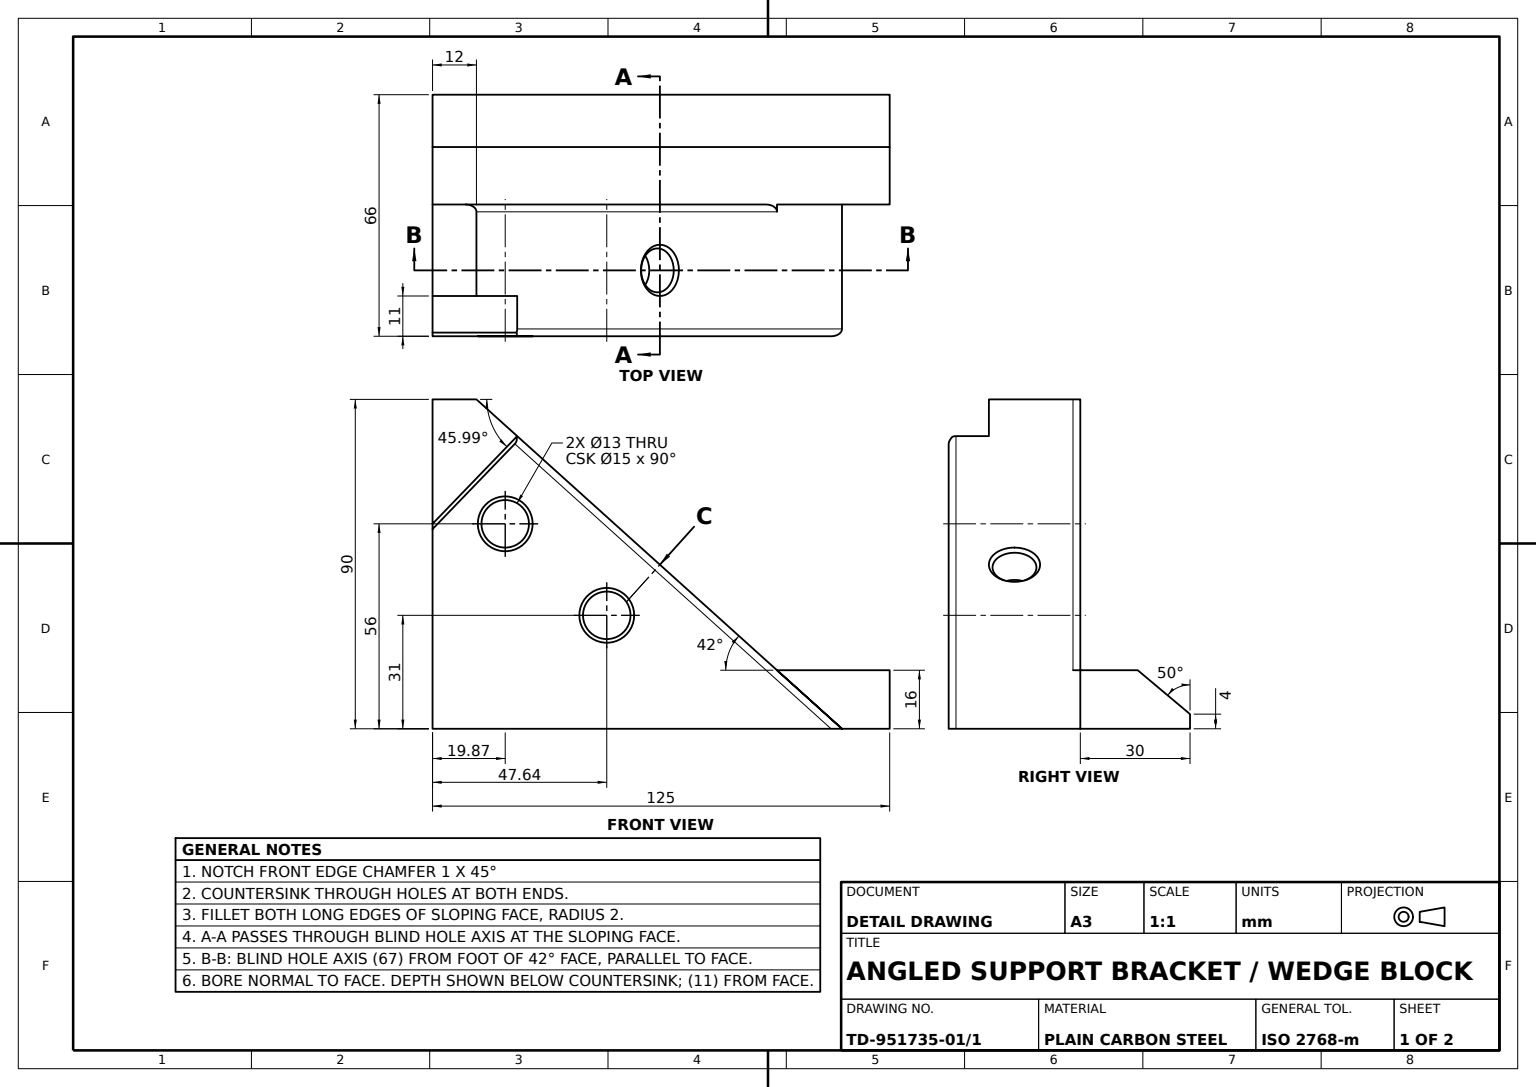
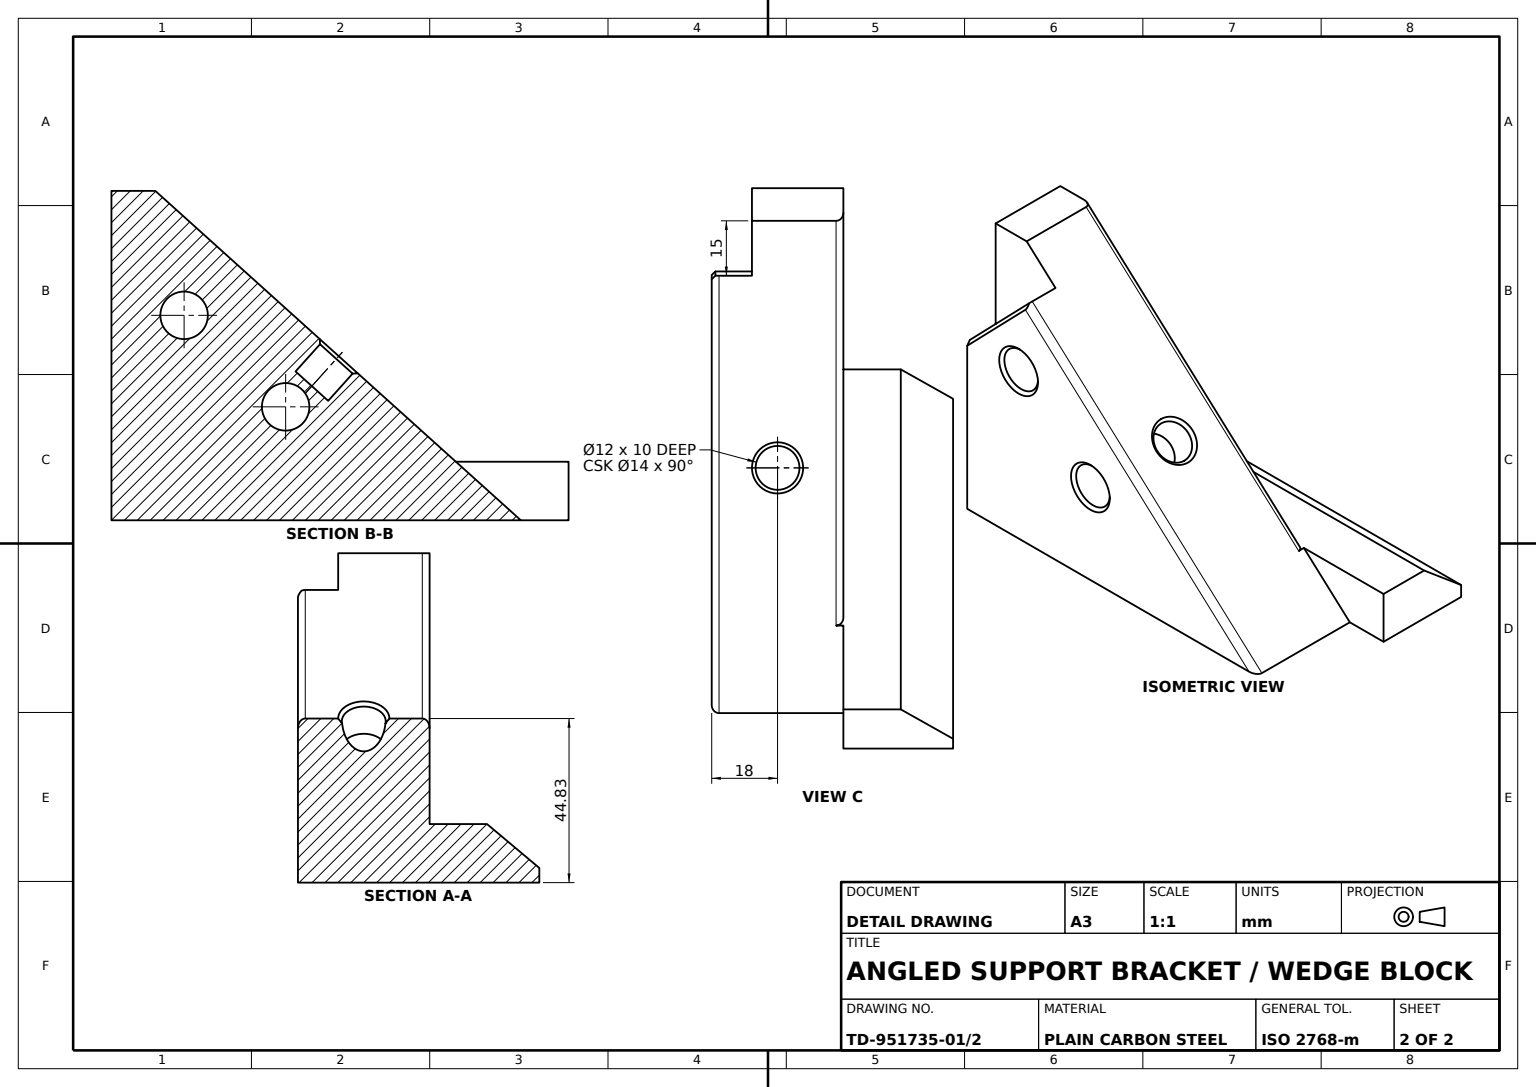
SolidWorks part; units mm, degrees
material "Plain Carbon Steel"
ref_plane "Front Plane" through (0, 0, 0) normal (0, 0, 1) x (1, 0, 0)
ref_plane "Top Plane" through (0, 0, 0) normal (0, 1, 0) x (1, 0, 0)
ref_plane "Right Plane" through (0, 0, 0) normal (1, 0, 0) x (0, 0, -1)
sketch "Bracket Profile Sketch" plane through (0, 0, 0) normal (0, 0, 1) x (1, 0, 0)
  line L0 (0, 0) -> (111.9551, 0)
  line L1 (111.9551, 0) -> (12, 90)
  line L2 (12, 90) -> (0, 90)
  line L3 (0, 90) -> (0, 0)
  dimension "D1" = 42
  dimension "D2" = 90
  dimension "D3" = 12
extrude "Triangular Bracket Body" add sketch "Bracket Profile Sketch" along normal mid plane 36
sketch "Rectangular Cut Sketch" plane through (0, 0, 18) normal (0, 0, 1) x (1, 0, 0)
  line L0 (23.1472, 79.963) -> (0, 56)
  line L1 (111.9551, 0) -> (12, 90) construction
  line L2 (0, 90) -> (0, 0) construction
  line L3 (0, 90) -> (0, 56)
  line L4 (0, 90) -> (12, 90)
  line L5 (12, 90) -> (23.1472, 79.963)
  dimension "D1" = 15
  dimension "D2" = 56
extrude "Rectangular Cut 15x56" cut sketch "Rectangular Cut Sketch" against normal blind 11
sketch "Hole Sketch" plane through (50.1263, 55.6709, 0) normal (0.6691, 0.7431, 0) x (0.7431, -0.6691, 0)
  line L0 (83.1989, -18) -> (83.1989, 18) construction
  circle A0 centre (16.1989, 0) radius 6
  dimension "D2" = 12
  dimension "D1" = 67
extrude "Hole Cut" cut sketch "Hole Sketch" against normal blind 11
sketch "Slide Rail Profile Sketch" plane through (0, 0, 0) normal (-1, 0, 0) x (0, 0, 1)
  line L0 (-18, 16) -> (-33.699, 16)
  line L1 (-18, 90) -> (-18, 0) construction
  line L2 (-33.699, 16) -> (-48, 4)
  line L3 (-48, 4) -> (-48, 0)
  line L4 (-48, 0) -> (-18, 0)
  line L5 (-18, 0) -> (-18, 16)
  dimension "D1" = 30
  dimension "D2" = 50
  dimension "D3" = 4
  dimension "D4" = 16
extrude "Slide Rail 125" add sketch "Slide Rail Profile Sketch" against normal blind 125
sketch "Rail Groove Sketch" plane through (0, 0, -18) normal (0, 0, -1) x (-1, 0, 0)
  line L0 (-125, 16) -> (0, 16) construction
  line L1 (-19.8713, 56) -> (-47.6366, 31) construction
  line L2 (-94.1853, 16) -> (-12, 90) construction
  line L3 (-94.1853, 16) -> (0, 16) construction
  circle A0 centre (-47.6366, 31) radius 6.5
  circle A1 centre (-19.8713, 56) radius 6.5
  dimension "D1" = 13
  dimension "D2" = 40
  dimension "D3" = 15
  dimension "D4" = 20
extrude "Rail Groove Cut" cut sketch "Rail Groove Sketch" against normal blind 125
chamfer "Rectangular Cut Chamfer 1mm" distance 1 angle 45 1 edges at (11.5736, 67.9815, 18)
chamfer "Hole and Groove Chamfer 1mm" distance 1 angle 45 5 edges at (41.1366, 31, -18) (13.3713, 56, -18) (54.1366, 31, 18) (26.3713, 56, 18) (57.7056, 48.8465, 0)
fillet "Body Edge Fillet R2 A" radius 2 1 edges at (53.0927, 53, -18)
fillet "Body Edge Fillet R2 B" radius 2 1 edges at (67.923, 39.6467, 18)
